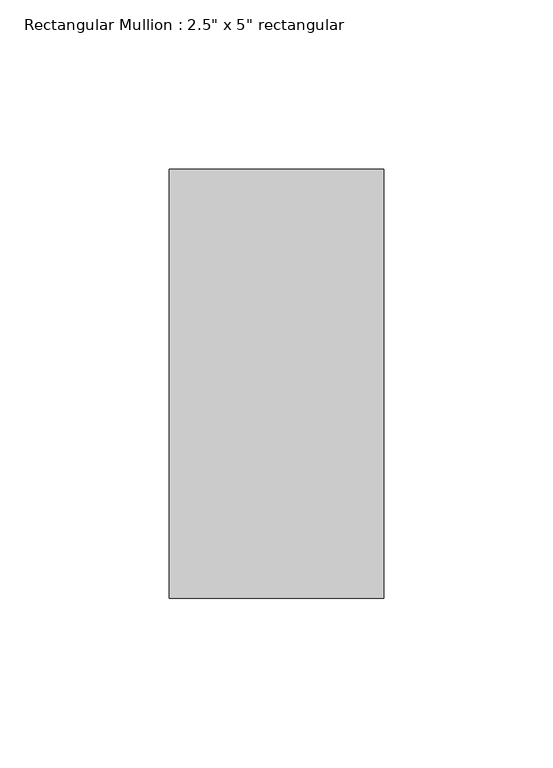
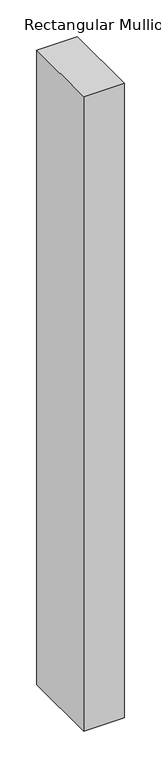
"""IFC4 building model written with IfcOpenShell, lengths in millimetres: member geometry."""

from ifc_helpers import new_model, si_unit, frame, origin, place, context, project, spatial, polyline, outline, extrude, source, transform, mapped, element, save


def member_9fa6ebbc(model_context):
    return source(origin(), model_context, "Body", "SweptSolid", [
        extrude(outline(polyline([(0.0, 63.5), (0.0, -63.5), (-63.5, -63.5), (-63.5, 63.5), (0.0, 63.5)])), frame((0.0, 0.0, -1052.4373156), z_axis=(0.0, 0.0, 1.0), x_axis=(1.0, 0.0, 0.0)), (0.0, 0.0, 1.0), 1052.4373156),
    ])


if __name__ == "__main__":
    model = new_model("IFC4")
    model_context = context("Model", 3, world=origin())
    ifc_project = project(units=[si_unit("LENGTHUNIT", "METRE", prefix="MILLI")], contexts=[model_context])
    site = spatial("IfcSite", under=ifc_project)
    building = spatial("IfcBuilding", under=site)
    placement = place(None, origin())
    member_shape = member_9fa6ebbc(model_context)
    element("IfcMember", 1, ObjectType="Rectangular Mullion : 2.5\" x 5\" rectangular", at=placement, inside=building, context=model_context, shape_type="MappedRepresentation", body=[
        mapped(member_shape, transform((0.0, 0.0, 0.0), x_axis=(1.0, 0.0, 0.0), y_axis=(0.0, 1.0, 0.0), z_axis=(0.0, 0.0, 1.0))),
    ])
    save(model, "model.ifc")

# Revit data of these elements
# Type "Rectangular Mullion : 2.5\" x 5\" rectangular"
#   built-in parameter 1007304 = 0.416667 (stored number, unit not read)
#   built-in parameter 1007301 = 0.104167 (stored number, unit not read)
#   built-in parameter 1007300 = 0.104167 (stored number, unit not read)
# Element 1 (IfcMember, "Rectangular Mullion : 2.5\" x 5\" rectangular")
#   Materials on its faces: "Aluminum"
# Materials
#   "Aluminum": class "Metal", colour RGB 247 247 247, transparency 0, Description = "Aluminum 6061", Cost = 0
